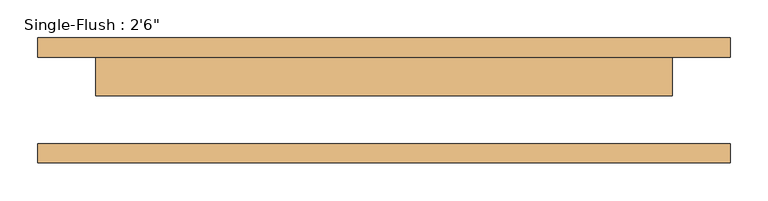
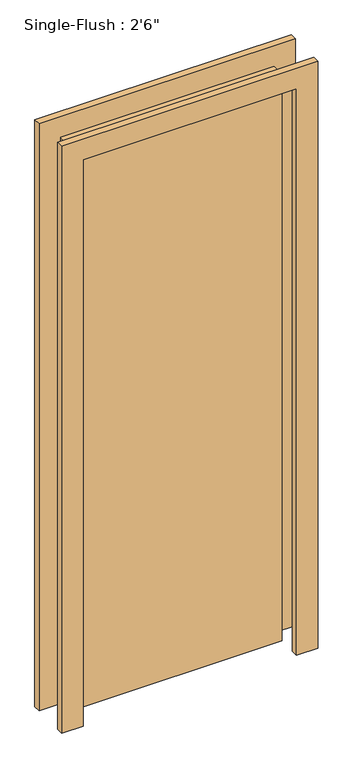
"""IFC4 building model written with IfcOpenShell, lengths in millimetres: door geometry."""

from ifc_helpers import new_model, si_unit, frame, origin, origin_with_axes, place, context, project, spatial, polyline, outline, extrude, source, transform, mapped, element, save


def door_214872d5(model_context):
    return source(origin(), model_context, "Body", "SweptSolid", [
        extrude(outline(polyline([(2209.8, -457.2), (0.0, -457.2), (0.0, -381.0), (2133.6, -381.0), (2133.6, 381.0), (0.0, 381.0), (0.0, 457.2), (2209.8, 457.2), (2209.8, -457.2)])), frame((0.0, 57.15, 0.0), z_axis=(0.0, 1.0, 0.0), x_axis=(0.0, 0.0, 1.0)), (0.0, 0.0, 1.0), 25.4),
        extrude(outline(polyline([(2209.8, 457.2), (2209.8, -457.2), (0.0, -457.2), (0.0, -381.0), (2133.6, -381.0), (2133.6, 381.0), (0.0, 381.0), (0.0, 457.2), (2209.8, 457.2)])), frame((0.0, -82.55, 0.0), z_axis=(0.0, 1.0, 0.0), x_axis=(0.0, 0.0, 1.0)), (0.0, 0.0, 1.0), 25.4),
        extrude(outline(polyline([(381.0, 6.35), (-381.0, 6.35), (-381.0, 57.15), (381.0, 57.15), (381.0, 6.35)])), origin_with_axes(), (0.0, 0.0, 1.0), 2133.6),
    ])


if __name__ == "__main__":
    model = new_model("IFC4")
    model_context = context("Model", 3, world=origin())
    ifc_project = project(units=[si_unit("LENGTHUNIT", "METRE", prefix="MILLI")], contexts=[model_context])
    site = spatial("IfcSite", under=ifc_project)
    building = spatial("IfcBuilding", under=site)
    placement = place(None, origin())
    door_shape = door_214872d5(model_context)
    element("IfcDoor", 1, ObjectType="Single-Flush : 2'6\"", at=placement, inside=building, context=model_context, shape_type="MappedRepresentation", body=[
        mapped(door_shape, transform((0.0, 0.0, 0.0), x_axis=(1.0, 0.0, 0.0), y_axis=(0.0, 1.0, 0.0), z_axis=(0.0, 0.0, 1.0))),
    ])
    save(model, "model.ifc")

# Revit data of these elements
# Type "Single-Flush : 2'6\""
#   Type Mark = "10"
#   Construction Type Id = "MDOOR"
#   Assembly Code = "C1020"
#   Analytic Construction = "Metal"
#   Thickness = 0' - 2"
#   Heat Transfer Coefficient (U) = 0.651978 BTU/(h·ft²·°F)
#   Height = 7' - 0"
#   Trim Projection Ext = 0' - 1"
#   Trim Projection Int = 0' - 1"
#   Trim Width = 0' - 3"
#   Width = 2' - 6"
#   Define Thermal Properties by = 1
#   Door Material = Door - Panel
#   Frame Material = Door - Frame
#   Visual Light Transmittance = 0
#   Solar Heat Gain Coefficient = 0
#   Function = (empty or 0)
#   Wall Closure = (empty or 0)
# Element 1 (IfcDoor, "Single-Flush : 2'6\"")
#   Materials on its faces: "Door - Frame", "Door - Panel"
# Materials
#   "Door - Panel": class "Wood", colour RGB 210 159 95, transparency 0, Cost = 0
#   "Door - Frame": colour RGB 118 70 51, transparency 0, Cost = 0
